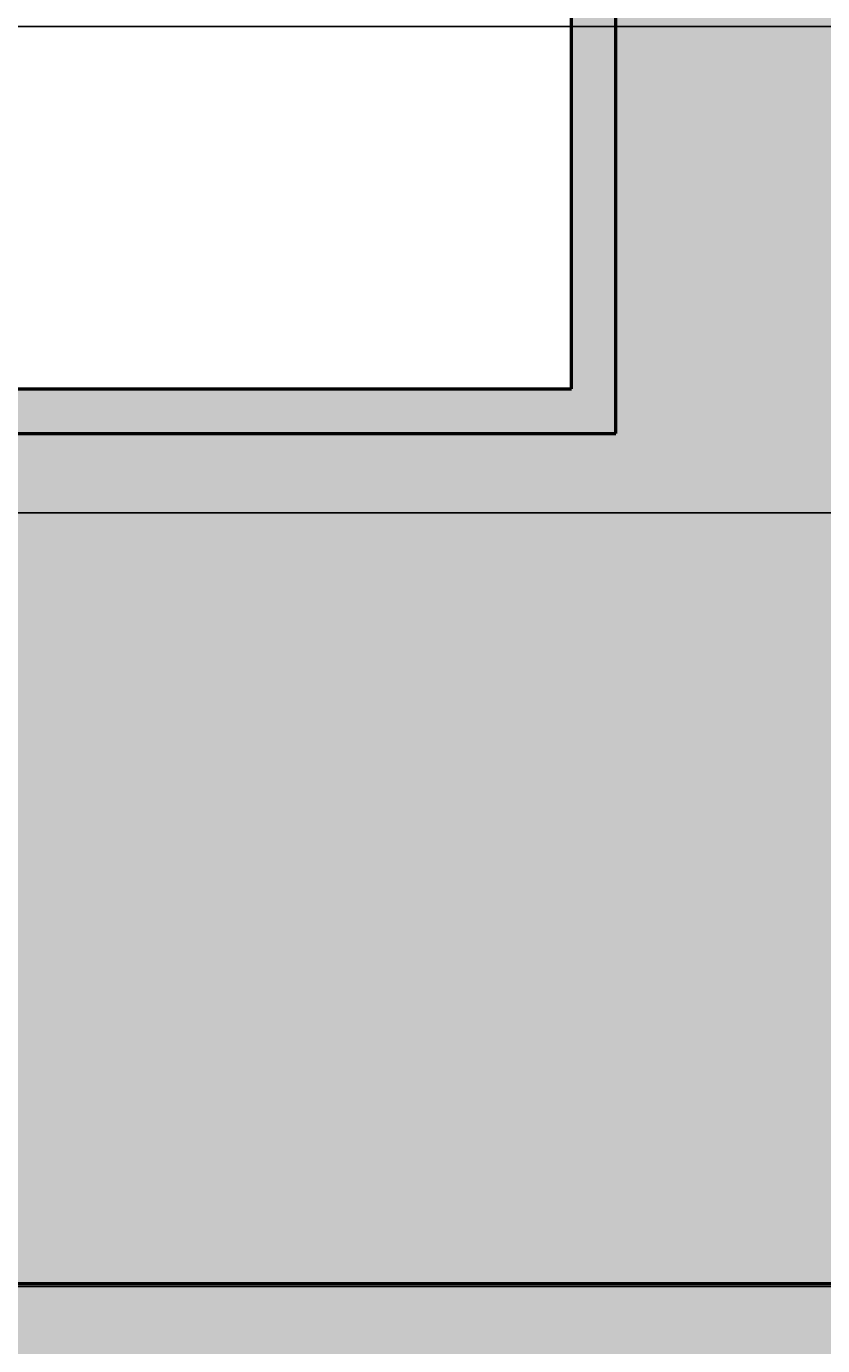
# Model space of a CAD drawing. Units: inches. Extents: x -12 to 334, y -10 to 186.
# Tile 8 of 77: x 24 to 42, y 79 to 109. Entities that reach past the tile are written whole.
import ezdxf

# ---------------------------------------------------------------- set-up
doc = ezdxf.new("R2010")
doc.units = ezdxf.units.IN
doc.header["$MEASUREMENT"] = 0
for name, color, linetype, lineweight in [('M-DIMS', 2, 'Continuous', 18), ('M-EQPM', 7, 'Continuous', 50), ('M-EQPM-PATT', 8, 'Continuous', 18)]:
    doc.layers.add(name, color=color, linetype=linetype, lineweight=lineweight)
doc.styles.get("Standard").update_dxf_attribs({"font": 'arial.ttf'})
doc.dimstyles.get("Standard").update_dxf_attribs({"dimtxt": 0.18, "dimasz": 0.18, "dimexe": 0.18, "dimexo": 0.0625, "dimgap": 0.09, "dimtad": 0, "dimtih": 1, "dimtoh": 1, "dimdec": 4, "dimzin": 0, "dimdsep": 46, "dimtxsty": 'Standard', "dimcen": 0.09, "dimadec": 0, "dimazin": 0, "dimtfac": 1, "dimtdec": 4, "dimtofl": 0, "dimtmove": 0, "dimatfit": 3, "dimfxl": 1, "dimtolj": 1, "dimtzin": 0, "dimarcsym": 0})

# ---------------------------------------------------------------- blocks, each defined once
blk = doc.blocks.new('*D1')
at = {"layer": 'Defpoints', "color": 0, "transparency": 16777216}
for p in [(281.426, 91.899), (3.376, 80.692), (281.426, 14.304)]:
    blk.add_point(p, dxfattribs=at)
at = {"layer": 'M-DIMS', "color": 0, "lineweight": -2, "transparency": 16777216}
for p, q in [((281.426, 91.836), (281.426, 14.124)), ((3.376, 80.629), (3.376, 14.124)), ((3.556, 14.304), (141.935, 14.304)), ((281.246, 14.304), (142.867, 14.304))]:
    blk.add_line(p, q, dxfattribs=at)
at = {"layer": 'M-DIMS', "color": 0, "transparency": 16777216}
for points in [[(3.556, 14.334), (3.556, 14.274), (3.376, 14.304)], [(281.246, 14.334), (281.246, 14.274), (281.426, 14.304)]]:
    blk.add_solid(points, dxfattribs=at)
at = {"layer": 'M-DIMS', "color": 0, "transparency": 16777216, "insert": (142.401, 14.304), "char_height": 0.18, "attachment_point": 5}
blk.add_mtext('\\A1;278.05', dxfattribs=at)
blk = doc.blocks.new('*D2')
at = {"layer": 'Defpoints', "color": 0, "transparency": 16777216}
for p in [(32.1, 169.385), (32.1, 127.708), (3.376, 80.692)]:
    blk.add_point(p, dxfattribs=at)
at = {"layer": 'M-DIMS', "color": 0, "lineweight": -2, "transparency": 16777216}
for p, q in [((3.376, 80.754), (3.376, 169.565)), ((3.556, 169.385), (17.274, 169.385)), ((31.92, 169.385), (18.203, 169.385)), ((32.1, 127.77), (32.1, 169.565))]:
    blk.add_line(p, q, dxfattribs=at)
at = {"layer": 'M-DIMS', "color": 0, "transparency": 16777216}
for points in [[(3.556, 169.415), (3.556, 169.355), (3.376, 169.385)], [(31.92, 169.415), (31.92, 169.355), (32.1, 169.385)]]:
    blk.add_solid(points, dxfattribs=at)
at = {"layer": 'M-DIMS', "color": 0, "transparency": 16777216, "insert": (17.738, 169.385), "char_height": 0.18, "attachment_point": 5}
blk.add_mtext('\\A1;28.724', dxfattribs=at)
blk = doc.blocks.new('*D8')
at = {"layer": 'Defpoints', "color": 0, "transparency": 16777216}
for p in [(-11.174, 127.708), (32.1, 127.708), (23.581, 100.896)]:
    blk.add_point(p, dxfattribs=at)
at = {"layer": 'M-DIMS', "color": 0, "lineweight": -2, "transparency": 16777216}
for p, q in [((32.038, 127.708), (-11.354, 127.708)), ((-11.174, 127.528), (-11.174, 114.484)), ((-11.174, 101.076), (-11.174, 114.12)), ((23.518, 100.896), (-11.354, 100.896))]:
    blk.add_line(p, q, dxfattribs=at)
at = {"layer": 'M-DIMS', "color": 0, "transparency": 16777216}
for points in [[(-11.204, 127.528), (-11.144, 127.528), (-11.174, 127.708)], [(-11.204, 101.076), (-11.144, 101.076), (-11.174, 100.896)]]:
    blk.add_solid(points, dxfattribs=at)
at = {"layer": 'M-DIMS', "color": 0, "transparency": 16777216, "insert": (-11.174, 114.302), "char_height": 0.18, "attachment_point": 5}
blk.add_mtext('\\A1;26.81', dxfattribs=at)
blk = doc.blocks.new('*D14')
at = {"layer": 'Defpoints', "color": 0, "transparency": 16777216}
for p in [(63.5, 109.058), (-11.174, 49.45), (64.207, 49.45)]:
    blk.add_point(p, dxfattribs=at)
at = {"layer": 'M-DIMS', "color": 0, "lineweight": -2, "transparency": 16777216}
for p, q in [((63.438, 109.058), (-11.354, 109.058)), ((-11.174, 108.878), (-11.174, 79.436)), ((-11.174, 49.63), (-11.174, 79.072)), ((64.144, 49.45), (-11.354, 49.45))]:
    blk.add_line(p, q, dxfattribs=at)
at = {"layer": 'M-DIMS', "color": 0, "transparency": 16777216}
for points in [[(-11.204, 108.878), (-11.144, 108.878), (-11.174, 109.058)], [(-11.204, 49.63), (-11.144, 49.63), (-11.174, 49.45)]]:
    blk.add_solid(points, dxfattribs=at)
at = {"layer": 'M-DIMS', "color": 0, "transparency": 16777216, "insert": (-11.174, 79.254), "char_height": 0.18, "attachment_point": 5}
blk.add_mtext('\\A1;59.61', dxfattribs=at)
blk = doc.blocks.new('*D35')
at = {"layer": 'Defpoints', "color": 0, "transparency": 16777216}
for p in [(216.428, 98.108), (-11.174, 61.105), (216.428, 61.105)]:
    blk.add_point(p, dxfattribs=at)
at = {"layer": 'M-DIMS', "color": 0, "lineweight": -2, "transparency": 16777216}
for p, q in [((216.365, 98.108), (-11.354, 98.108)), ((-11.174, 97.928), (-11.174, 79.788)), ((-11.174, 61.285), (-11.174, 79.424)), ((216.365, 61.105), (-11.354, 61.105))]:
    blk.add_line(p, q, dxfattribs=at)
at = {"layer": 'M-DIMS', "color": 0, "transparency": 16777216}
for points in [[(-11.204, 97.928), (-11.144, 97.928), (-11.174, 98.108)], [(-11.204, 61.285), (-11.144, 61.285), (-11.174, 61.105)]]:
    blk.add_solid(points, dxfattribs=at)
at = {"layer": 'M-DIMS', "color": 0, "transparency": 16777216, "insert": (-11.174, 79.606), "char_height": 0.18, "attachment_point": 5}
blk.add_mtext('\\A1;37', dxfattribs=at)
blk = doc.blocks.new('*D39')
at = {"layer": 'Defpoints', "color": 0, "transparency": 16777216}
for p in [(279.726, 80.692), (-11.174, 45.854), (269.381, 45.854)]:
    blk.add_point(p, dxfattribs=at)
at = {"layer": 'M-DIMS', "color": 0, "lineweight": -2, "transparency": 16777216}
for p, q in [((279.664, 80.692), (-11.354, 80.692)), ((-11.174, 80.512), (-11.174, 63.455)), ((-11.174, 46.034), (-11.174, 63.091)), ((269.318, 45.854), (-11.354, 45.854))]:
    blk.add_line(p, q, dxfattribs=at)
at = {"layer": 'M-DIMS', "color": 0, "transparency": 16777216}
for points in [[(-11.204, 80.512), (-11.144, 80.512), (-11.174, 80.692)], [(-11.204, 46.034), (-11.144, 46.034), (-11.174, 45.854)]]:
    blk.add_solid(points, dxfattribs=at)
at = {"layer": 'M-DIMS', "color": 0, "transparency": 16777216, "insert": (-11.174, 63.273), "char_height": 0.18, "attachment_point": 5}
blk.add_mtext('\\A1;34.84', dxfattribs=at)

msp = doc.modelspace()

# ---------------------------------------------------------------- hatches: boundary and pattern name
at = {"layer": 'M-EQPM-PATT'}
h = msp.add_hatch(color=256, dxfattribs=at)
h.set_gradient(color1=(99, 100, 102), color2=(99, 100, 102), tint=1)
h.paths.add_polyline_path([(4.3766, 80.754, -0.4132606), (23.5807, 99.8958), (37.1002, 99.8958), (37.1002, 127.7078), (32.1002, 127.7078), (32.1002, 125.2078), (36.1002, 125.2078), (36.1002, 100.8958), (23.5807, 100.8958, 1), (23.5807, 60.4872), (36.1002, 60.4872), (36.1002, 36.1752), (32.1002, 36.1752), (32.1002, 33.6752), (37.1002, 33.6752), (37.1002, 61.4872), (23.5807, 61.4872, -0.384914), (4.4744, 78.754), (72.9244, 78.754), (72.9244, 69.6117), (75.9244, 69.6117), (75.9244, 89.8963), (72.9244, 89.8963), (72.9244, 80.754)])
h.paths.add_polyline_path([(54.1002, 125.2078), (58.1002, 125.2078), (58.1002, 127.7078), (53.1002, 127.7078), (53.1002, 99.8958), (64.5, 99.8958), (64.5, 109.0583), (63.5, 109.0583), (63.5, 100.8958), (54.1002, 100.8958)], flags=17)
h.paths.add_polyline_path([(53.1002, 33.6752), (58.1002, 33.6752), (58.1002, 36.1752), (54.1002, 36.1752), (54.1002, 60.4872), (64.2068, 60.4872), (64.2068, 49.4497), (87.8879, 49.4497), (87.8879, 55.3205), (104.8919, 55.3205), (104.8919, 30.8541), (99.8919, 30.8541), (99.8919, 28.8541), (105.8919, 28.8541), (105.8919, 56.3205), (87.8879, 56.3205), (87.8879, 63.6117), (86.8879, 63.6117), (86.8879, 50.4497), (65.0061, 50.4497), (65.0061, 63.6117), (64.5, 63.6117), (64.5, 61.4872), (53.1002, 61.4872)])
h.paths.add_polyline_path([(121.8919, 28.8541), (121.8919, 30.8541), (116.8919, 30.8541), (116.8919, 45.8541), (209.6965, 45.8541), (209.9204, 46.8541), (115.8919, 46.8541), (115.8919, 28.8541)])
h.paths.add_polyline_path([(221.5761, 32.8541), (216.5761, 32.8541), (216.5761, 30.8541), (222.5761, 30.8541), (222.5761, 46.8541), (209.9204, 46.8541), (209.6965, 45.8541), (221.5761, 45.8541)])
h.paths.add_polyline_path([(233.5761, 45.8541), (249.8485, 45.8541), (249.3759, 46.8541), (232.5761, 46.8541), (232.5761, 30.8541), (238.5761, 30.8541), (238.5761, 32.8541), (233.5761, 32.8541)])
h = msp.add_hatch(color=256, dxfattribs=at)
h.set_gradient(color1=(205, 32, 39), color2=(205, 32, 39), tint=1)
h.paths.add_polyline_path([(64.5, 80.754), (64.5, 89.8963), (226.6083, 89.8963, -1), (226.6083, 69.6117), (64.5, 69.6117), (64.5, 78.754), (4.4744, 78.754, 0.384914), (23.5807, 61.4872), (37.1002, 61.4872), (37.1002, 33.6752), (53.1002, 33.6752), (53.1002, 61.4872), (64.5, 61.4872), (64.5, 63.6117), (226.6083, 63.6117, 1), (226.6083, 95.8963), (64.5, 95.8963), (64.5, 99.8958), (53.1002, 99.8958), (53.1002, 127.7078), (37.1002, 127.7078), (37.1002, 99.8958), (23.5807, 99.8958, 0.4132606), (4.3766, 80.754)])
h.paths.add_polyline_path([(64.5, 91.8963), (64.5, 93.8963), (226.6083, 93.8963, -1), (226.6083, 65.6117), (64.5, 65.6117), (64.5, 67.6117), (226.6083, 67.6117, 1), (226.6083, 91.8963)], flags=16)

# ---------------------------------------------------------------- linework, layer by layer
at = {"layer": 'M-EQPM'}
for p, q in [((37.1002, 99.8958), (37.1002, 127.7078)), ((36.1002, 100.8958), (36.1002, 125.2078)), ((72.9244, 80.754), (4.3766, 80.754))]:
    msp.add_line(p, q, dxfattribs=at)
for points in [[(36.1002, 60.4872), (23.5807, 60.4872, -1), (23.5807, 100.8958), (36.1002, 100.8958)], [(4.3766, 80.754, -0.4132606), (23.5807, 99.8958), (37.1002, 99.8958)]]:
    msp.add_lwpolyline(points, format="xyb", dxfattribs=at)

# ---------------------------------------------------------------- dimensions: what is measured, and where the dimension line sits
at = {"layer": 'M-DIMS'}
for base, p2, override, picture, middle in [((32.1002, 169.3845), (32.1002, 127.7078), {"dimdec": 3, "dimlfac": 1, "dimrnd": 0, "dimzin": 0, "dimdsep": 46, "dimlunit": 2}, '*D2', (17.7383, 169.3845)), ((281.4256, 14.3041), (281.4256, 91.8988), {"dimdec": 2, "dimlfac": 1, "dimrnd": 0, "dimzin": 0, "dimdsep": 46, "dimlunit": 2}, '*D1', (142.401, 14.3041))]:
    dim = msp.add_linear_dim(base=base, p1=(3.3765, 80.6915), p2=p2, dimstyle='Standard', override=override, dxfattribs=at)
    dim.commit()
    dim.dimension.update_dxf_attribs({"geometry": picture, "text_midpoint": middle})
for base, p1, p2, override, picture, middle in [((-11.1736, 127.7078), (23.5807, 100.8958), (32.1002, 127.7078), {"dimdec": 2, "dimlfac": 1, "dimrnd": 0, "dimzin": 0, "dimdsep": 46, "dimlunit": 2}, '*D8', (-11.1735, 114.3018)), ((-11.1736, 49.4497), (63.5, 109.0583), (64.2068, 49.4497), {"dimdec": 2, "dimlfac": 1, "dimrnd": 0, "dimzin": 0, "dimdsep": 46, "dimlunit": 2}, '*D14', (-11.1735, 79.254)), ((-11.1736, 61.1045), (216.4278, 98.1081), (216.4278, 61.1045), {"dimdec": 0, "dimlfac": 1, "dimrnd": 0, "dimzin": 0, "dimdsep": 46, "dimlunit": 2}, '*D35', (-11.1735, 79.6063)), ((-11.1736, 45.8541), (279.7263, 80.6915), (269.3808, 45.8541), {"dimdec": 2, "dimlfac": 1, "dimrnd": 0, "dimzin": 0, "dimdsep": 46, "dimlunit": 2}, '*D39', (-11.1735, 63.2728))]:
    dim = msp.add_linear_dim(base=base, p1=p1, p2=p2, angle=90, dimstyle='Standard', override=override, dxfattribs=at)
    dim.commit()
    dim.dimension.update_dxf_attribs({"geometry": picture, "text_midpoint": middle})

doc.saveas('drawing.dxf')
